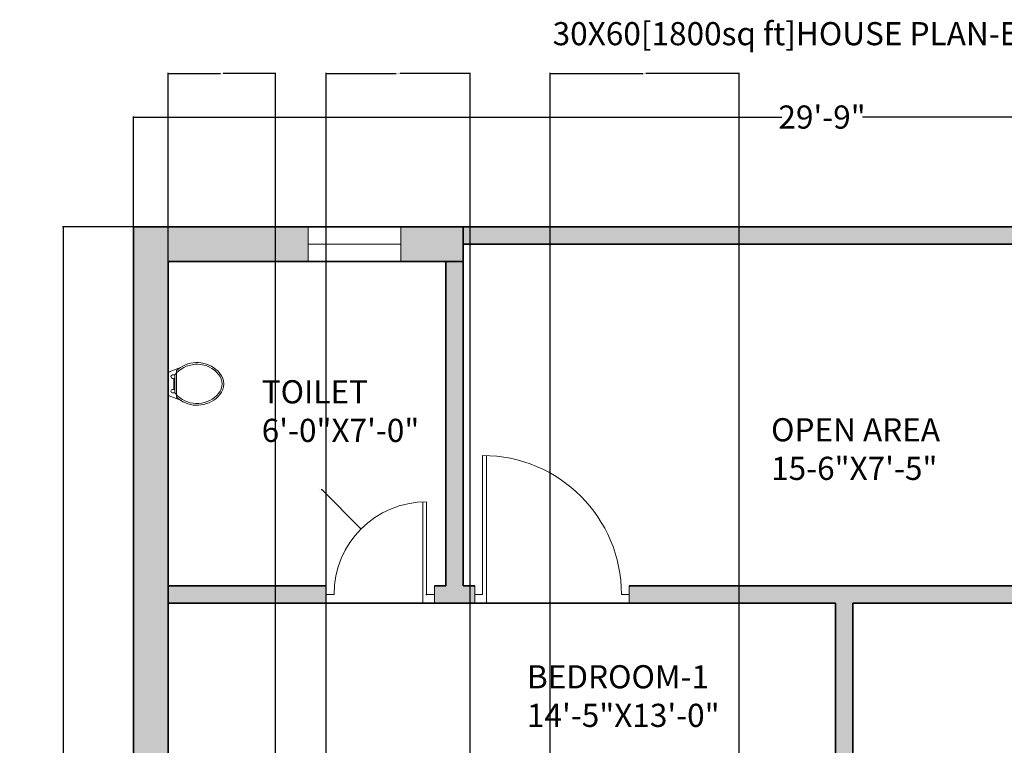
# Model space of a CAD drawing. Units: inches. Extents: x -15 to 423, y -713 to 71.
# Tile 10 of 24: x -4 to 251, y -117 to 71. Entities that reach past the tile are written whole.
import ezdxf

# ---------------------------------------------------------------- set-up
doc = ezdxf.new("R2010")
doc.units = ezdxf.units.IN
doc.header["$MEASUREMENT"] = 0
for name, color, linetype, lineweight in [('A-ANNO-DIMS', 2, 'Continuous', 18), ('A-ANNO-TEXT', 7, 'Continuous', 18), ('A-AREA-IDEN', 7, 'Continuous', 18), ('A-DOOR', 3, 'Continuous', 18), ('A-GLAZ', 5, 'Continuous', 18), ('A-WALL', 7, 'Continuous', 35), ('A-WALL-PATT', 8, 'Continuous', 13), ('WC-Detail_dwgmodels.com', 251, 'Continuous', 13), ('WC-Outline_dwgmodels.com', 250, 'Continuous', 18)]:
    doc.layers.add(name, color=color, linetype=linetype, lineweight=lineweight)
doc.styles.get("Standard").update_dxf_attribs({"font": 'arial.ttf'})
doc.dimstyles.get("Standard").update_dxf_attribs({"dimtxt": 0.18, "dimasz": 0.18, "dimexe": 0.18, "dimexo": 0.0625, "dimgap": 0.09, "dimtad": 0, "dimtih": 1, "dimtoh": 1, "dimdec": 0, "dimzin": 0, "dimdsep": 46, "dimlunit": 3, "dimtxsty": 'Standard', "dimcen": 0.09, "dimadec": 0, "dimazin": 0, "dimtfac": 1, "dimtdec": 0, "dimtofl": 0, "dimtmove": 0, "dimatfit": 3, "dimfxl": 1, "dimtolj": 1, "dimtzin": 0, "dimarcsym": 0})

# ---------------------------------------------------------------- blocks, each defined once
blk = doc.blocks.new('*D7')
at = {"layer": 'A-ANNO-DIMS', "color": 0, "lineweight": -2, "transparency": 16777216}
for p, q in [((25.08, 17.56), (25.08, 46.15)), ((25.26, 45.97), (193.13, 45.97)), ((381.9, 45.97), (214.03, 45.97)), ((382.08, 17.56), (382.08, 46.15))]:
    blk.add_line(p, q, dxfattribs=at)
at = {"layer": 'A-ANNO-DIMS', "color": 0, "transparency": 16777216}
for points in [[(25.26, 46), (25.26, 45.94), (25.08, 45.97)], [(381.9, 46), (381.9, 45.94), (382.08, 45.97)]]:
    blk.add_solid(points, dxfattribs=at)
at = {"layer": 'Defpoints', "color": 0, "transparency": 16777216}
for p in [(25.08, 45.97), (25.08, 17.5), (382.08, 17.5)]:
    blk.add_point(p, dxfattribs=at)
at = {"layer": 'A-ANNO-DIMS', "color": 0, "transparency": 16777216, "insert": (203.58, 45.97), "char_height": 6, "attachment_point": 5}
blk.add_mtext('\\A1;29\'-9"', dxfattribs=at)
blk = doc.blocks.new('*D8')
at = {"layer": 'A-ANNO-DIMS', "color": 0, "lineweight": -2, "transparency": 16777216}
for p, q in [((25.02, 17.5), (6.72, 17.5)), ((6.9, 17.32), (6.9, -193.09)), ((6.9, -409.82), (6.9, -199.41)), ((34.02, -410), (6.72, -410))]:
    blk.add_line(p, q, dxfattribs=at)
at = {"layer": 'A-ANNO-DIMS', "color": 0, "transparency": 16777216}
for points in [[(6.87, 17.32), (6.93, 17.32), (6.9, 17.5)], [(6.87, -409.82), (6.93, -409.82), (6.9, -410)]]:
    blk.add_solid(points, dxfattribs=at)
at = {"layer": 'Defpoints', "color": 0, "transparency": 16777216}
for p in [(25.08, 17.5), (6.9, -410), (34.08, -410)]:
    blk.add_point(p, dxfattribs=at)
at = {"layer": 'A-ANNO-DIMS', "color": 0, "transparency": 16777216, "insert": (6.9, -196.25), "char_height": 6, "attachment_point": 5}
blk.add_mtext('\\A1;35\'-8"', dxfattribs=at)
blk = doc.blocks.new('WINDOW-24IN')
for p, q in [((9, 24), (0, 24)), ((0, 24), (0, 0)), ((4.5, 0), (4.5, 24)), ((9, 0), (9, 24)), ((0, 0), (9, 0))]:
    blk.add_line(p, q)
blk = doc.blocks.new('DOOR-24IN-JAMB4_5')
for p, q in [((25, 0), (25, 26.25)), ((26, 2.25), (26, 26.25)), ((0, 2.25), (0, 4.5)), ((28, 4.5), (28, 0)), ((2, 2.25), (0, 2.25)), ((0, 2.25), (0, 0)), ((28, 2.25), (26, 2.25))]:
    blk.add_line(p, q)
blk.add_arc((26, 2.25), 24, 90, 180)
blk = doc.blocks.new('DOOR-36IN-JAMB4_5')
for p, q in [((2, 2.25), (2, 38.25)), ((3, 0), (3, 38.25)), ((0, 4.5), (0, 0)), ((40, 2.25), (40, 4.5)), ((0, 2.25), (2, 2.25)), ((38, 2.25), (40, 2.25)), ((40, 2.25), (40, 0))]:
    blk.add_line(p, q)
blk.add_arc((2, 2.25), 36, 0, 90)
blk = doc.blocks.new('*D37')
at = {"layer": 'A-ANNO-DIMS', "color": 0, "lineweight": -2, "transparency": 16777216}
for p, q in [((34.08, -396.44), (34.08, 57.43)), ((34.26, 57.25), (47.65, 57.25)), ((61.7, 57.25), (48.31, 57.25)), ((61.88, -396.44), (61.88, 57.43))]:
    blk.add_line(p, q, dxfattribs=at)
at = {"layer": 'A-ANNO-DIMS', "color": 0, "transparency": 16777216}
for points in [[(34.26, 57.28), (34.26, 57.22), (34.08, 57.25)], [(61.7, 57.28), (61.7, 57.22), (61.88, 57.25)]]:
    blk.add_solid(points, dxfattribs=at)
at = {"layer": 'Defpoints', "color": 0, "transparency": 16777216}
for p in [(61.88, 57.25), (34.08, -396.5), (61.88, -396.5)]:
    blk.add_point(p, dxfattribs=at)
at = {"layer": 'A-ANNO-DIMS', "color": 0, "transparency": 16777216, "insert": (47.98, 57.25), "char_height": 0.18, "attachment_point": 5}
blk.add_mtext('\\A1;2\'-4"', dxfattribs=at)
blk = doc.blocks.new('*D39')
at = {"layer": 'A-ANNO-DIMS', "color": 0, "lineweight": -2, "transparency": 16777216}
for p, q in [((75.05, -253.53), (75.05, 57.43)), ((75.23, 57.25), (93.19, 57.25)), ((112.22, 57.25), (94.26, 57.25)), ((112.4, -253.53), (112.4, 57.43))]:
    blk.add_line(p, q, dxfattribs=at)
at = {"layer": 'A-ANNO-DIMS', "color": 0, "transparency": 16777216}
for points in [[(75.23, 57.28), (75.23, 57.22), (75.05, 57.25)], [(112.22, 57.28), (112.22, 57.22), (112.4, 57.25)]]:
    blk.add_solid(points, dxfattribs=at)
at = {"layer": 'Defpoints', "color": 0, "transparency": 16777216}
for p in [(112.4, 57.25), (75.05, -253.59), (112.4, -253.59)]:
    blk.add_point(p, dxfattribs=at)
at = {"layer": 'A-ANNO-DIMS', "color": 0, "transparency": 16777216, "insert": (93.72, 57.25), "char_height": 0.18, "attachment_point": 5}
blk.add_mtext('\\A1;3\'-1 1/2"', dxfattribs=at)
blk = doc.blocks.new('*D42')
at = {"layer": 'A-ANNO-DIMS', "color": 0, "lineweight": -2, "transparency": 16777216}
for p, q in [((133.08, -409.94), (133.08, 57.43)), ((133.26, 57.25), (157.25, 57.25)), ((181.9, 57.25), (157.91, 57.25)), ((182.08, -409.94), (182.08, 57.43))]:
    blk.add_line(p, q, dxfattribs=at)
at = {"layer": 'A-ANNO-DIMS', "color": 0, "transparency": 16777216}
for points in [[(133.26, 57.28), (133.26, 57.22), (133.08, 57.25)], [(181.9, 57.28), (181.9, 57.22), (182.08, 57.25)]]:
    blk.add_solid(points, dxfattribs=at)
at = {"layer": 'Defpoints', "color": 0, "transparency": 16777216}
for p in [(182.08, 57.25), (133.08, -410), (182.08, -410)]:
    blk.add_point(p, dxfattribs=at)
at = {"layer": 'A-ANNO-DIMS', "color": 0, "transparency": 16777216, "insert": (157.58, 57.25), "char_height": 0.18, "attachment_point": 5}
blk.add_mtext('\\A1;4\'-1"', dxfattribs=at)
blk = doc.blocks.new('*D44')
at = {"layer": 'A-ANNO-DIMS', "color": 0, "lineweight": -2, "transparency": 16777216}
for p, q in [((73.75, -50.6), (73.93, -50.6)), ((73.93, -50.6), (83.98, -60.65)), ((100.99, -77.75), (101.17, -77.75)), ((101.08, -77.84), (101.08, -77.66))]:
    blk.add_line(p, q, dxfattribs=at)
at = {"layer": 'A-ANNO-DIMS', "color": 0, "transparency": 16777216}
blk.add_solid([(84, -60.63), (83.96, -60.67), (84.11, -60.78)], dxfattribs=at)
at = {"layer": 'Defpoints', "color": 0, "transparency": 16777216}
for p in [(84.11, -60.78), (101.08, -77.75)]:
    blk.add_point(p, dxfattribs=at)
at = {"layer": 'A-ANNO-DIMS', "color": 0, "transparency": 16777216, "insert": (73.33, -50.6), "char_height": 0.18, "attachment_point": 5}
blk.add_mtext('\\A1;R2\'-0"', dxfattribs=at)

msp = doc.modelspace()

# ---------------------------------------------------------------- hatches: boundary and pattern name
at = {"layer": 'A-WALL-PATT'}
h = msp.add_hatch(color=256, dxfattribs=at)
h.dxf.hatch_style = 1
h.paths.add_polyline_path([(34.08, -349.58), (25.08, -349.58), (25.08, -431), (34.08, -431)])
h.paths.add_polyline_path([(34.08, -467), (25.08, -467), (25.08, -673), (34.08, -673)])
h.paths.add_polyline_path([(373.08, -668.5), (182.08, -668.5), (182.08, -673), (373.08, -673)])
h.paths.add_polyline_path([(253.2, -597.5), (191.08, -597.5), (191.08, -594.5), (182.08, -594.5), (182.08, -606.5), (253.2, -606.5)])
h.paths.add_polyline_path([(373.08, -597.5), (313.2, -597.5), (313.2, -606.5), (373.08, -606.5)])
h.paths.add_polyline_path([(382.08, -545.55), (373.08, -545.55), (373.08, -673), (382.08, -673)])
h.paths.add_polyline_path([(139.08, -488), (34.08, -488), (34.08, -497), (139.08, -497), (139.08, -492.5)])
h.paths.add_polyline_path([(139.08, -396.5), (128.58, -396.5), (128.58, -352.79), (124.08, -352.79), (124.08, -396.5), (34.08, -396.5), (34.08, -410), (139.08, -410), (139.08, -403.25)])
h.paths.add_polyline_path([(191.08, -396.5), (179.08, -396.5), (179.08, -410), (182.08, -410), (182.08, -488), (179.08, -488), (179.08, -497), (182.08, -497), (182.08, -501.43), (191.08, -501.43)])
h.paths.add_polyline_path([(373.08, -396.5), (253.08, -396.5), (253.08, -393.5), (248.58, -393.5), (248.58, -401), (284.58, -401), (284.58, -404), (289.08, -404), (289.08, -401), (373.08, -401)])
h.paths.add_polyline_path([(373.08, -449), (289.08, -449), (289.08, -432), (286.83, -432), (284.58, -432), (284.58, -453.5), (373.08, -453.5)])
h.paths.add_polyline_path([(382.08, -344.27), (373.08, -344.27), (373.08, -413.68), (382.08, -413.68)])
h.paths.add_polyline_path([(382.08, -437.68), (373.08, -437.68), (373.08, -485.55), (382.08, -485.55)])
h.paths.add_polyline_path([(34.08, -188.26), (25.08, -188.26), (25.08, -289.58), (34.08, -289.58)])
h.paths.add_polyline_path([(164.08, -236), (34.08, -236), (34.08, -240.5), (124.08, -240.5), (124.08, -293.12), (128.58, -293.12), (128.58, -240.5), (164.08, -240.5), (164.08, -238.25)])
h.paths.add_polyline_path([(373.08, -236), (242.58, -236), (242.58, -238.25), (242.58, -240.5), (248.58, -240.5), (248.58, -353.5), (250.83, -353.5), (253.08, -353.5), (253.08, -240.5), (373.08, -240.5)])
h.paths.add_polyline_path([(382.08, -190.86), (373.08, -190.86), (373.08, -284.27), (382.08, -284.27)])
h.paths.add_polyline_path([(211.58, -80), (253.58, -80), (253.58, -77.75), (253.58, -75.5), (153.58, -75.5), (153.58, -77.75), (153.58, -80), (207.08, -80), (207.08, -236), (204.08, -236), (204.08, -240.5), (214.58, -240.5), (214.58, -236), (211.58, -236)])
h.paths.add_polyline_path([(34.08, 8.5), (70.36, 8.5), (70.36, 17.5), (25.08, 17.5), (25.08, -128.26), (34.08, -128.26)])
h.paths.add_polyline_path([(110.58, 17.5), (94.36, 17.5), (94.36, 8.5), (110.58, 8.5)])
h.paths.add_polyline_path([(296.58, 17.5), (110.58, 17.5), (110.58, 13), (296.58, 13)])
h.paths.add_polyline_path([(110.58, 8.5), (106.08, 8.5), (106.08, -75.5), (103.08, -75.5), (103.08, -80), (113.58, -80), (113.58, -77.75), (113.58, -75.5), (110.58, -75.5)])
h.paths.add_polyline_path([(75.08, -75.5), (34.08, -75.5), (34.08, -80), (75.08, -80), (75.08, -77.75)])
h.paths.add_polyline_path([(343.09, 17.5), (296.58, 17.5), (296.58, 13), (296.58, 8.5), (343.09, 8.5)])
h.paths.add_polyline_path([(304.08, -75.5), (301.08, -75.5), (301.08, 8.5), (296.58, 8.5), (296.58, -75.5), (293.58, -75.5), (293.58, -80), (304.08, -80)])
h.paths.add_polyline_path([(382.08, 17.5), (367.09, 17.5), (367.09, 8.5), (373.08, 8.5), (373.08, -130.86), (382.08, -130.86)])
h.paths.add_polyline_path([(373.08, -75.5), (332.08, -75.5), (332.08, -77.75), (332.08, -80), (373.08, -80)])

# ---------------------------------------------------------------- linework, layer by layer
at = {"layer": 'A-DOOR'}
msp.add_line((113.58, -80), (113.58, -77.75), dxfattribs=at)
at = {"layer": 'A-WALL'}
for p, q in [((25.08, 17.5), (25.08, -673)), ((25.08, 17.5), (382.08, 17.5)), ((110.58, 17.5), (110.58, -75.5)), ((110.58, 13), (296.58, 13)), ((34.08, 8.5), (110.58, 8.5)), ((34.08, 8.5), (34.08, -673)), ((106.08, 8.5), (106.08, -75.5)), ((34.08, -75.5), (75.08, -75.5)), ((103.08, -75.5), (106.08, -75.5)), ((110.58, -75.5), (113.58, -75.5)), ((153.58, -75.5), (253.58, -75.5)), ((34.08, -80), (207.08, -80)), ((207.08, -80), (207.08, -236)), ((211.58, -80), (211.58, -236)), ((211.58, -80), (373.08, -80))]:
    msp.add_line(p, q, dxfattribs=at)
at = {"layer": 'WC-Detail_dwgmodels.com'}
for p, q in [((36.27, -20.35), (36.27, -19.74)), ((36.27, -26.65), (36.27, -26.04))]:
    msp.add_line(p, q, dxfattribs=at)
for points in [[(35.83, -20.85, -0.022712), (36.27, -20.35, -0.162618)], [(36.27, -19.74, -0.040937), (37.26, -18.96, -0.163732)], [(35.83, -20.85), (35.23, -20.85, 1), (35.23, -21.77), (35.54, -21.77)], [(35.83, -23.19), (35.83, -20.85, -0.476108)], [(35.83, -25.54), (35.23, -25.54, -1), (35.23, -24.62), (35.54, -24.62)], [(35.83, -23.19), (35.83, -25.54, 0.022712)], [(35.83, -25.54, 0.022712), (36.27, -26.04, 0.162618)], [(36.27, -26.65, 0.040937), (37.26, -27.43, 0.163732)]]:
    msp.add_lwpolyline(points, format="xyb", dxfattribs=at)
for points in [[(35.54, -21.77), (35.54, -24.62)], [(35.54, -21.77), (35.83, -21.77)], [(35.54, -24.62), (35.83, -24.62)]]:
    msp.add_lwpolyline(points, dxfattribs=at)
at = {"layer": 'WC-Outline_dwgmodels.com'}
for p in [(36.27, -20.35), (36.27, -26.04)]:
    msp.add_line(p, (36.27, -23.19), dxfattribs=at)
for points in [[(37.26, -18.96, -0.383919), (47.51, -20.47, -0.163732), (48.55, -23.19, -0.359733)], [(34.08, -23.19), (34.08, -20.43, -0.31031), (34.31, -20.09), (37.26, -18.96, -0.209071)], [(36.27, -20.35, -0.448546), (47.17, -20.75, -0.162618), (48.12, -23.19, -0.470877)], [(34.08, -23.19), (34.08, -25.96, 0.31031), (34.31, -26.3), (37.26, -27.43, 0.209071)], [(36.57, -26.33, 0.431639), (47.17, -25.64, 0.162618), (48.12, -23.19, 0.470877)], [(37.26, -27.43, 0.383919), (47.51, -25.91, 0.163732), (48.55, -23.19, 0.359733)], [(36.27, -26.04, 0.014165), (36.57, -26.33, 0.162618)]]:
    msp.add_lwpolyline(points, format="xyb", dxfattribs=at)

# ---------------------------------------------------------------- block references
at = {"layer": 'A-DOOR'}
for name, p in [('DOOR-36IN-JAMB4_5', (113.58, -80)), ('DOOR-24IN-JAMB4_5', (75.08, -80))]:
    msp.add_blockref(name, p, dxfattribs=at)
at = {"layer": 'A-GLAZ', "rotation": 269.9999999999998}
msp.add_blockref('WINDOW-24IN', (70.36, 17.5), dxfattribs=at)

# ---------------------------------------------------------------- texts
at = {"layer": 'A-ANNO-TEXT', "insert": (133.75, 70.58), "char_height": 6, "attachment_point": 1}
msp.add_mtext('30X60[1800sq ft]HOUSE PLAN-EAST FACE-FP1062', dxfattribs=at)
at = {"layer": 'A-AREA-IDEN', "char_height": 6, "attachment_point": 1}
for s, insert in [('TOILET\\P6\'-0"X7\'-0"', (58.33, -22.24)), ('OPEN AREA\\P15-6"X7\'-5"', (190.37, -32.08)), ('BEDROOM-1\\P14\'-5"X13\'-0"', (127.09, -96.1))]:
    msp.add_mtext(s, dxfattribs=dict(at, insert=insert))

# ---------------------------------------------------------------- dimensions: what is measured, and where the dimension line sits
at = {"layer": 'A-ANNO-DIMS'}
for base, p1, p2, override, picture, middle in [((61.88, 57.25), (34.08, -396.5), (61.88, -396.5), {"dimdec": 1, "dimlfac": 1, "dimrnd": 0, "dimzin": 1, "dimdsep": 46, "dimlunit": 4, "dimfrac": 2}, '*D37', (47.98, 57.25)), ((112.3972, 57.2501), (75.0509, -253.5887), (112.3972, -253.5887), {"dimdec": 1, "dimlfac": 1, "dimrnd": 0, "dimzin": 1, "dimdsep": 46, "dimlunit": 4, "dimfrac": 2}, '*D39', (93.724, 57.2501)), ((182.08, 57.25), (133.08, -410), (182.08, -410), {"dimdec": 1, "dimlfac": 1, "dimrnd": 0, "dimzin": 1, "dimdsep": 46, "dimlunit": 4, "dimfrac": 2}, '*D42', (157.58, 57.25)), ((25.08, 45.97), (382.08, 17.5), (25.08, 17.5), {"dimtxt": 6, "dimclrd": 0, "dimclre": 0, "dimclrt": 0}, '*D7', (203.58, 45.97))]:
    dim = msp.add_linear_dim(base=base, p1=p1, p2=p2, dimstyle='Standard', override=override, dxfattribs=at)
    dim.commit()
    dim.dimension.update_dxf_attribs({"geometry": picture, "text_midpoint": middle})
dim = msp.add_linear_dim(base=(6.9041327, -409.99989936), p1=(25.08055573, 17.50010064), p2=(34.08055573, -409.99989936), angle=90, dimstyle='Standard', override={"dimtxt": 6, "dimclrd": 0, "dimclre": 0, "dimclrt": 0}, dxfattribs=at)
dim.commit()
dim.dimension.update_dxf_attribs({"geometry": '*D8', "text_midpoint": (6.9041327, -196.24989936)})
dim = msp.add_radius_dim(center=(101.08, -77.75), mpoint=(84.11, -60.78), dimstyle='Standard', override={"dimdec": 1, "dimlfac": 1, "dimrnd": 0, "dimzin": 1, "dimdsep": 46, "dimlunit": 4, "dimfrac": 2}, dxfattribs=at)
dim.commit()
dim.dimension.update_dxf_attribs({"geometry": '*D44', "text_midpoint": (73.33, -50.6), "dimtype": 164})

doc.saveas('drawing.dxf')
